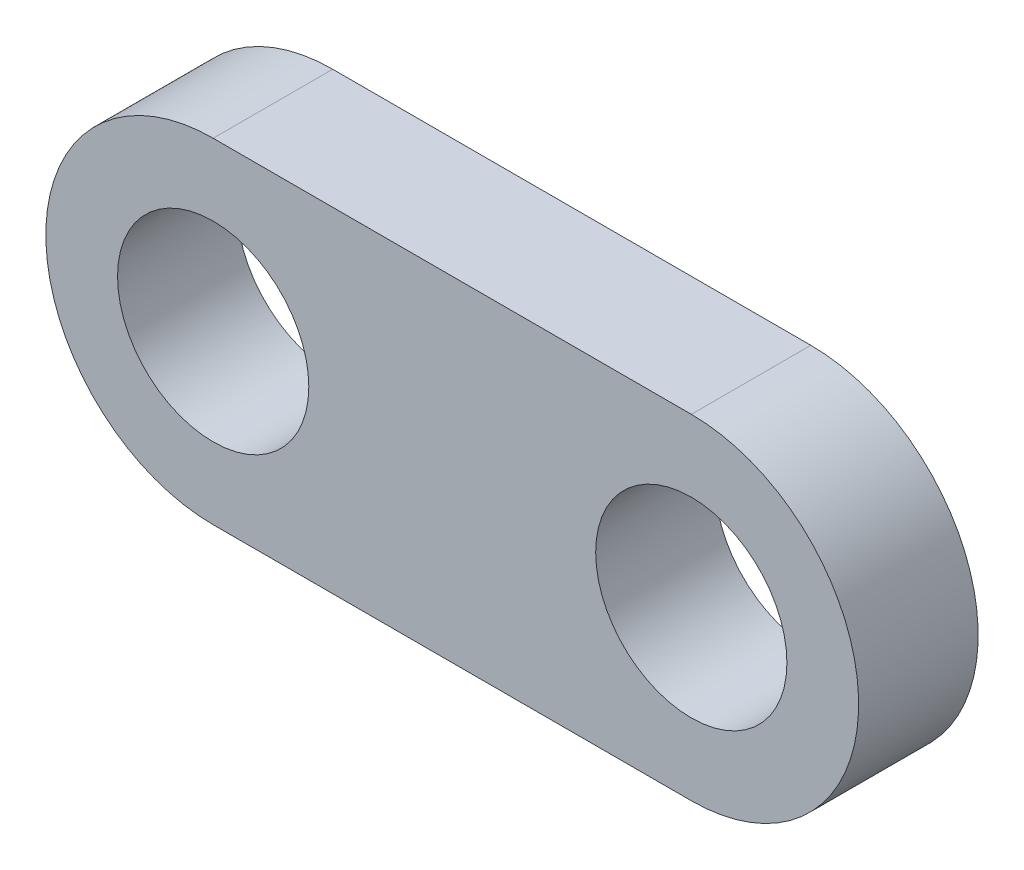
from build123d import *

# Parameters (mm, degrees)
LINK_PROFILE_SKETCH_R = 4
LINK_PLATE_5MM_DEPTH  = 2.5


with BuildPart() as part:
    # Link Profile Sketch → Link Plate 5mm (new, symmetric)
    with BuildSketch(Plane.XY):
        with BuildLine():
            Line((-10, 7), (10, 7))
            ThreePointArc((10, 7), (17, 0), (10, -7))
            Line((10, -7), (-10, -7))
            ThreePointArc((-10, -7), (-17, 0), (-10, 7))
        make_face()
        with Locations((-10, 0)):
            Circle(LINK_PROFILE_SKETCH_R, mode=Mode.SUBTRACT)
        with Locations((10, 0)):
            Circle(LINK_PROFILE_SKETCH_R, mode=Mode.SUBTRACT)
    extrude(amount=LINK_PLATE_5MM_DEPTH, both=True)


solid = part.part
